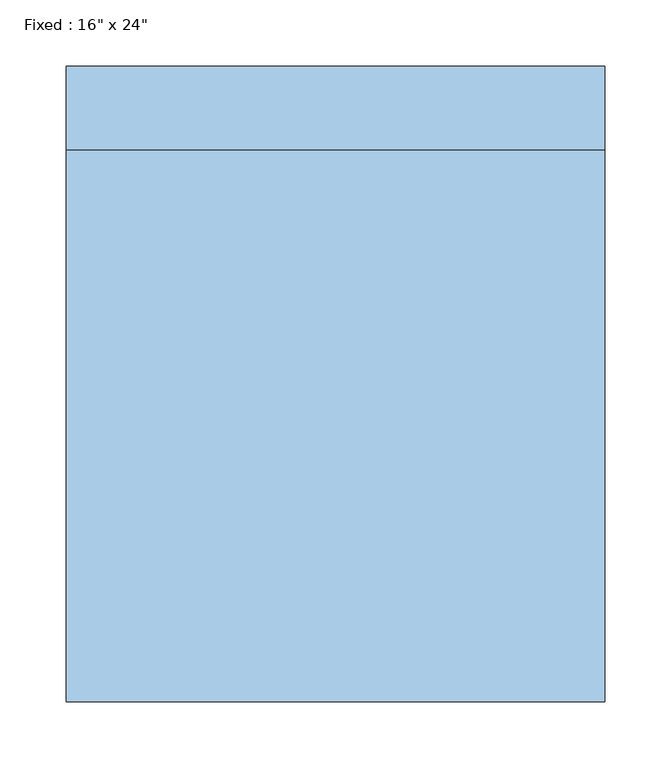
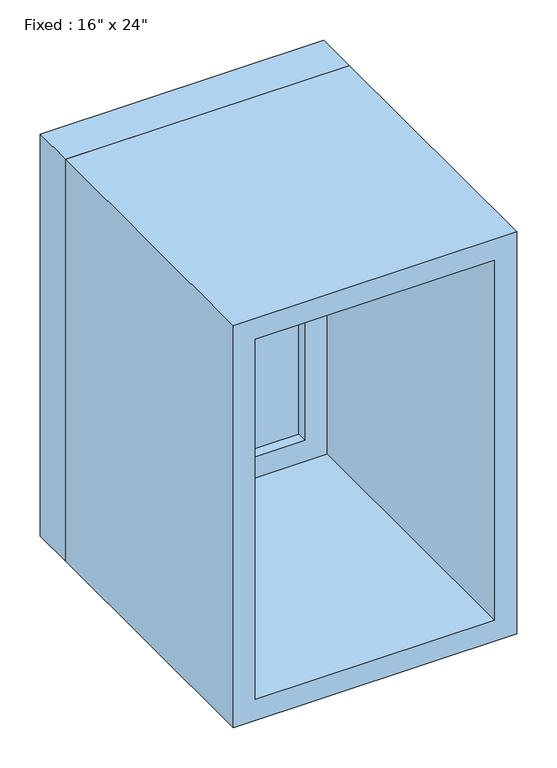
"""IFC4 building model written with IfcOpenShell, lengths in millimetres: window geometry."""

from ifc_helpers import new_model, si_unit, frame, origin, place, context, project, spatial, polyline, outline, extrude, source, transform, mapped, element, save


def window_8bd8a12f(model_context):
    return source(origin(), model_context, "Body", "SweptSolid", [
        extrude(outline(polyline([(101.6, 192.1472809), (-177.8, 192.1472809), (-177.8, 204.8472809), (101.6, 204.8472809), (101.6, 192.1472809)])), frame((0.0, 0.0, 977.9), z_axis=(0.0, 0.0, 1.0), x_axis=(1.0, 0.0, 0.0)), (0.0, 0.0, 1.0), 482.6),
        extrude(outline(polyline([(1504.95, -222.25), (933.45, -222.25), (933.45, 146.05), (1504.95, 146.05), (1504.95, -222.25)]), holes=[polyline([(1460.5, -177.8), (1460.5, 101.6), (977.9, 101.6), (977.9, -177.8), (1460.5, -177.8)])]), frame((0.0, 176.2722809, 0.0), z_axis=(0.0, 1.0, 0.0), x_axis=(0.0, 0.0, 1.0)), (0.0, 0.0, 1.0), 44.45),
        extrude(outline(polyline([(1524.0, -241.3), (914.4, -241.3), (914.4, 165.1), (1524.0, 165.1), (1524.0, -241.3)]), holes=[polyline([(1492.25, -209.55), (1492.25, 133.35), (946.15, 133.35), (946.15, -209.55), (1492.25, -209.55)])]), frame((0.0, -239.7722809, 0.0), z_axis=(0.0, 1.0, 0.0), x_axis=(0.0, 0.0, 1.0)), (0.0, 0.0, 1.0), 416.0445618),
        extrude(outline(polyline([(1524.0, 165.1), (1524.0, -241.3), (914.4, -241.3), (914.4, 165.1), (1524.0, 165.1)]), holes=[polyline([(1504.95, 146.05), (933.45, 146.05), (933.45, -222.25), (1504.95, -222.25), (1504.95, 146.05)])]), frame((0.0, 176.2722809, 0.0), z_axis=(0.0, 1.0, 0.0), x_axis=(0.0, 0.0, 1.0)), (0.0, 0.0, 1.0), 63.5),
    ])


if __name__ == "__main__":
    model = new_model("IFC4")
    model_context = context("Model", 3, world=origin())
    ifc_project = project(units=[si_unit("LENGTHUNIT", "METRE", prefix="MILLI")], contexts=[model_context])
    site = spatial("IfcSite", under=ifc_project)
    building = spatial("IfcBuilding", under=site)
    placement = place(None, origin())
    window_shape = window_8bd8a12f(model_context)
    element("IfcWindow", 1, ObjectType="Fixed : 16\" x 24\"", at=placement, inside=building, context=model_context, shape_type="MappedRepresentation", body=[
        mapped(window_shape, transform((0.0, 0.0, 0.0), x_axis=(1.0, 0.0, 0.0), y_axis=(0.0, 1.0, 0.0), z_axis=(0.0, 0.0, 1.0))),
    ])
    save(model, "model.ifc")

# Revit data of these elements
# Type "Fixed : 16\" x 24\""
#   Type Mark = "4"
#   Construction Type Id = "GSP4R"
#   Assembly Code = "B2020100"
#   Analytic Construction = "1/8 in Pilkington single glazing"
#   Visual Light Transmittance = 0.9
#   Solar Heat Gain Coefficient = 0.78
#   Heat Transfer Coefficient (U) = 0.6496 BTU/(h·ft²·°F)
#   Height = 2' - 0"
#   Default Sill Height = 3' - 0"
#   Width = 1' - 4"
#   Window Inset = 0' - 0 3/4"
#   Define Thermal Properties by = 1
#   Glass Pane Material = Glass
#   Sash Material = Sash
#   Wall Closure = (empty or 0)
# Element 1 (IfcWindow, "Fixed : 16\" x 24\"")
#   Materials on its faces: "Sash", "Glass"
# Materials
#   "Glass": class "Glass", colour RGB 0 128 192, transparency 0.75, Description = "Soda Lime Glass", Cost = 0
#   "Sash": class "Wood", colour RGB 224 178 126, transparency 0
